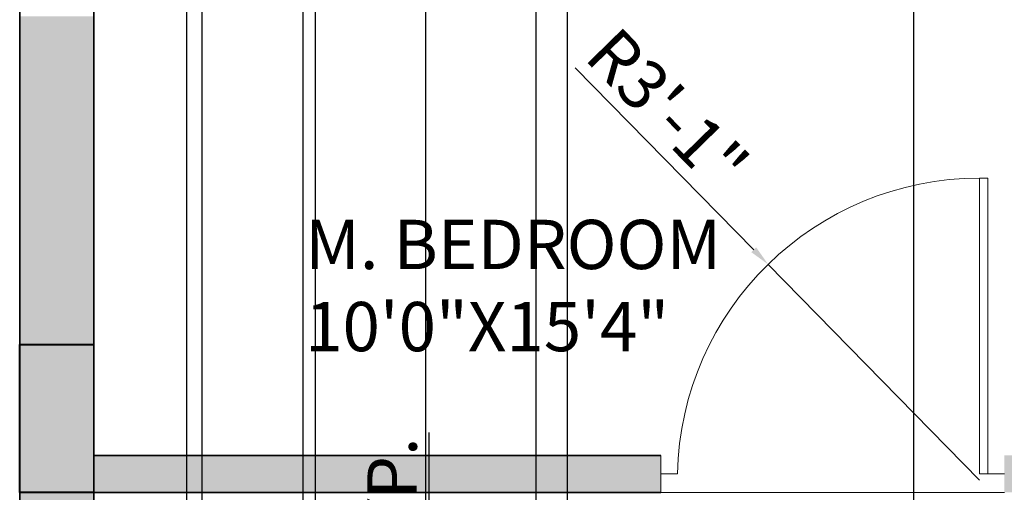
# Model space of a CAD drawing. Units: inches. Extents: x 2656 to 9931, y 1941 to 3068.
# Tile 5 of 46: x 2743 to 2863, y 2426 to 2484. Entities that reach past the tile are written whole.
import ezdxf

# ---------------------------------------------------------------- set-up
doc = ezdxf.new("R2010")
doc.units = ezdxf.units.IN
for name, color, linetype, lineweight in [('A-ANNO-DIMS', 2, 'Continuous', 18), ('A-AREA-IDEN', 7, 'Continuous', 18), ('A-COLS', 7, 'Continuous', 40), ('A-COLS-PATT', 146, 'Continuous', 13), ('A-DOOR', 3, 'Continuous', 18), ('A-WALL', 7, 'Continuous', 35), ('A-WALL-PATT', 251, 'Continuous', 13)]:
    doc.layers.add(name, color=color, linetype=linetype, lineweight=lineweight)
doc.styles.get("Standard").update_dxf_attribs({"font": 'arial.ttf'})
doc.dimstyles.new('ISO-25', dxfattribs={"dimtxt": 6, "dimasz": 2.5, "dimexe": 1.25, "dimexo": 0.625, "dimtad": 1, "dimdec": 0, "dimlunit": 3, "dimtxsty": 'Standard', "dimcen": 2.5, "dimadec": 0, "dimazin": 0, "dimtfac": 1, "dimtdec": 0, "dimtmove": 0, "dimatfit": 3, "dimfxl": 1, "dimarcsym": 0})

# ---------------------------------------------------------------- blocks, each defined once
blk = doc.blocks.new('DOOR-BEDROOM-DINING')
for p, q in [((39.78, 38.25), (38.78, 38.25)), ((38.78, 38.25), (38.78, 2.25)), ((39.78, 2.25), (39.78, 38.25)), ((0.03, 2.25), (2.03, 2.25)), ((38.78, 2.25), (39.78, 2.25)), ((41.78, 2.25), (39.78, 2.25)), ((0.03, 0), (41.78, 0))]:
    blk.add_line(p, q)
blk.add_arc((38.78, 1.5), 36.75, 90, 178.8304)
blk = doc.blocks.new('*D31')
at = {"layer": 'A-ANNO-DIMS', "color": 0, "lineweight": -2, "transparency": 16777216}
for p, q in [((2753.36, 2502.15), (2753.36, 2488.23)), ((2841.98, 2502.15), (2841.98, 2488.23)), ((2755.86, 2489.48), (2839.48, 2489.48)), ((2841.98, 2489.48), (2952.35, 2489.48))]:
    blk.add_line(p, q, dxfattribs=at)
at = {"layer": 'A-ANNO-DIMS', "color": 0, "transparency": 16777216}
for points in [[(2755.86, 2489.89), (2755.86, 2489.06), (2753.36, 2489.48)], [(2839.48, 2489.89), (2839.48, 2489.06), (2841.98, 2489.48)]]:
    blk.add_solid(points, dxfattribs=at)
at = {"layer": 'Defpoints', "color": 0, "transparency": 16777216}
for p in [(2753.36, 2502.77), (2841.98, 2502.77), (2841.98, 2489.48)]:
    blk.add_point(p, dxfattribs=at)
at = {"layer": 'A-ANNO-DIMS', "color": 0, "transparency": 16777216, "insert": (2898.41, 2493.21), "char_height": 6, "attachment_point": 5}
blk.add_mtext('DOUBLE BED 7\'-4 1/2" TYP.', dxfattribs=at)
blk = doc.blocks.new('*D62')
at = {"layer": 'A-ANNO-DIMS', "color": 0, "lineweight": -2, "transparency": 16777216}
for p, q in [((2792.93, 2374.42), (2792.93, 2433.38)), ((2791.71, 2374.42), (2794.18, 2374.42)), ((2792.93, 2365.48), (2792.93, 2371.92)), ((2791.71, 2362.98), (2794.18, 2362.98))]:
    blk.add_line(p, q, dxfattribs=at)
at = {"layer": 'A-ANNO-DIMS', "color": 0, "transparency": 16777216}
for points in [[(2792.52, 2371.92), (2793.35, 2371.92), (2792.93, 2374.42)], [(2792.52, 2365.48), (2793.35, 2365.48), (2792.93, 2362.98)]]:
    blk.add_solid(points, dxfattribs=at)
at = {"layer": 'Defpoints', "color": 0, "transparency": 16777216}
for p in [(2791.08, 2374.42), (2792.93, 2374.42), (2791.08, 2362.98)]:
    blk.add_point(p, dxfattribs=at)
at = {"layer": 'A-ANNO-DIMS', "color": 0, "transparency": 16777216, "insert": (2789.21, 2405.15), "char_height": 6, "attachment_point": 5, "rotation": 90}
blk.add_mtext('0\'-11 1/2" TYP.', dxfattribs=at)
blk = doc.blocks.new('*D113')
at = {"layer": 'A-ANNO-DIMS', "color": 0, "lineweight": -2, "transparency": 16777216}
for p, q in [((2752.16, 2300.73), (2752.16, 2674.45)), ((2809.77, 2300.73), (2809.77, 2674.45)), ((2754.66, 2673.2), (2807.27, 2673.2))]:
    blk.add_line(p, q, dxfattribs=at)
at = {"layer": 'A-ANNO-DIMS', "color": 0, "transparency": 16777216}
for points in [[(2754.66, 2673.62), (2754.66, 2672.78), (2752.16, 2673.2)], [(2807.27, 2673.62), (2807.27, 2672.78), (2809.77, 2673.2)]]:
    blk.add_solid(points, dxfattribs=at)
at = {"layer": 'Defpoints', "color": 0, "transparency": 16777216}
for p in [(2809.77, 2673.2), (2752.16, 2300.1), (2809.77, 2300.1)]:
    blk.add_point(p, dxfattribs=at)
at = {"layer": 'A-ANNO-DIMS', "color": 0, "transparency": 16777216, "insert": (2780.96, 2676.93), "char_height": 6, "attachment_point": 5}
blk.add_mtext('4\'-9 1/2"', dxfattribs=at)
blk = doc.blocks.new('*D114')
at = {"layer": 'A-ANNO-DIMS', "color": 0, "lineweight": -2, "transparency": 16777216}
for p, q in [((2809.77, 2300.73), (2809.77, 2674.45)), ((2851.88, 2300.73), (2851.88, 2674.45)), ((2812.27, 2673.2), (2849.38, 2673.2))]:
    blk.add_line(p, q, dxfattribs=at)
at = {"layer": 'A-ANNO-DIMS', "color": 0, "transparency": 16777216}
for points in [[(2812.27, 2673.62), (2812.27, 2672.78), (2809.77, 2673.2)], [(2849.38, 2673.62), (2849.38, 2672.78), (2851.88, 2673.2)]]:
    blk.add_solid(points, dxfattribs=at)
at = {"layer": 'Defpoints', "color": 0, "transparency": 16777216}
for p in [(2851.88, 2673.2), (2809.77, 2300.1), (2851.88, 2300.1)]:
    blk.add_point(p, dxfattribs=at)
at = {"layer": 'A-ANNO-DIMS', "color": 0, "transparency": 16777216, "insert": (2830.82, 2676.89), "char_height": 6, "attachment_point": 5}
blk.add_mtext('3\'-6"', dxfattribs=at)
blk = doc.blocks.new('*D129')
at = {"layer": 'A-ANNO-DIMS', "color": 0, "lineweight": -2, "transparency": 16777216}
for p, q in [((2752.16, 2601.15), (2752.16, 2009.27)), ((2777.59, 2557.74), (2777.59, 2009.27)), ((2754.66, 2010.52), (2775.09, 2010.52)), ((2777.59, 2010.52), (2811.37, 2010.52))]:
    blk.add_line(p, q, dxfattribs=at)
at = {"layer": 'A-ANNO-DIMS', "color": 0, "transparency": 16777216}
for points in [[(2754.66, 2010.94), (2754.66, 2010.11), (2752.16, 2010.52)], [(2775.09, 2010.94), (2775.09, 2010.11), (2777.59, 2010.52)]]:
    blk.add_solid(points, dxfattribs=at)
at = {"layer": 'Defpoints', "color": 0, "transparency": 16777216}
for p in [(2752.16, 2601.77), (2777.59, 2558.37), (2777.59, 2010.52)]:
    blk.add_point(p, dxfattribs=at)
at = {"layer": 'A-ANNO-DIMS', "color": 0, "transparency": 16777216, "insert": (2795.73, 2014.25), "char_height": 6, "attachment_point": 5}
blk.add_mtext('2\'-1 1/2"', dxfattribs=at)
blk = doc.blocks.new('*D132')
at = {"layer": 'A-ANNO-DIMS', "color": 0, "lineweight": -2, "transparency": 16777216}
for p, q in [((2763.47, 2366.56), (2763.47, 2674.45)), ((2805.96, 2366.56), (2805.96, 2674.45)), ((2765.97, 2673.2), (2803.46, 2673.2))]:
    blk.add_line(p, q, dxfattribs=at)
at = {"layer": 'A-ANNO-DIMS', "color": 0, "transparency": 16777216}
for points in [[(2765.97, 2673.62), (2765.97, 2672.78), (2763.47, 2673.2)], [(2803.46, 2673.62), (2803.46, 2672.78), (2805.96, 2673.2)]]:
    blk.add_solid(points, dxfattribs=at)
at = {"layer": 'Defpoints', "color": 0, "transparency": 16777216}
for p in [(2805.96, 2673.2), (2763.47, 2365.93), (2805.96, 2365.93)]:
    blk.add_point(p, dxfattribs=at)
at = {"layer": 'A-ANNO-DIMS', "color": 0, "transparency": 16777216, "insert": (2784.72, 2676.93), "char_height": 6, "attachment_point": 5}
blk.add_mtext('3\'-6 1/2"', dxfattribs=at)
blk = doc.blocks.new('*D134')
at = {"layer": 'A-ANNO-DIMS', "color": 0, "lineweight": -2, "transparency": 16777216}
for p, q in [((2752.16, 2300.73), (2752.16, 2674.45)), ((2763.47, 2347.43), (2763.47, 2674.45)), ((2754.66, 2673.2), (2760.97, 2673.2)), ((2763.47, 2673.2), (2801.81, 2673.2))]:
    blk.add_line(p, q, dxfattribs=at)
at = {"layer": 'A-ANNO-DIMS', "color": 0, "transparency": 16777216}
for points in [[(2754.66, 2673.62), (2754.66, 2672.78), (2752.16, 2673.2)], [(2760.97, 2673.62), (2760.97, 2672.78), (2763.47, 2673.2)]]:
    blk.add_solid(points, dxfattribs=at)
at = {"layer": 'Defpoints', "color": 0, "transparency": 16777216}
for p in [(2763.47, 2673.2), (2763.47, 2346.81), (2752.16, 2300.1)]:
    blk.add_point(p, dxfattribs=at)
at = {"layer": 'A-ANNO-DIMS', "color": 0, "transparency": 16777216, "insert": (2783.89, 2676.93), "char_height": 6, "attachment_point": 5}
blk.add_mtext('0\'-11 1/2"', dxfattribs=at)
blk = doc.blocks.new('*D136')
at = {"layer": 'A-ANNO-DIMS', "color": 0, "lineweight": -2, "transparency": 16777216}
for p, q in [((2765.36, 2375.04), (2765.36, 2674.45)), ((2779.14, 2375.04), (2779.14, 2674.45)), ((2767.86, 2673.2), (2776.64, 2673.2)), ((2779.14, 2673.2), (2798.28, 2673.2))]:
    blk.add_line(p, q, dxfattribs=at)
at = {"layer": 'A-ANNO-DIMS', "color": 0, "transparency": 16777216}
for points in [[(2767.86, 2673.62), (2767.86, 2672.78), (2765.36, 2673.2)], [(2776.64, 2673.62), (2776.64, 2672.78), (2779.14, 2673.2)]]:
    blk.add_solid(points, dxfattribs=at)
at = {"layer": 'Defpoints', "color": 0, "transparency": 16777216}
for p in [(2779.14, 2673.2), (2765.36, 2374.42), (2779.14, 2374.42)]:
    blk.add_point(p, dxfattribs=at)
at = {"layer": 'A-ANNO-DIMS', "color": 0, "transparency": 16777216, "insert": (2789.96, 2676.84), "char_height": 6, "attachment_point": 5}
blk.add_mtext('1\'-2"', dxfattribs=at)
blk = doc.blocks.new('*D137')
at = {"layer": 'A-ANNO-DIMS', "color": 0, "lineweight": -2, "transparency": 16777216}
for p, q in [((2779.14, 2375.04), (2779.14, 2674.45)), ((2792.52, 2375.04), (2792.52, 2674.45)), ((2781.64, 2673.2), (2790.02, 2673.2)), ((2792.52, 2673.2), (2825.63, 2673.2))]:
    blk.add_line(p, q, dxfattribs=at)
at = {"layer": 'A-ANNO-DIMS', "color": 0, "transparency": 16777216}
for points in [[(2781.64, 2673.62), (2781.64, 2672.78), (2779.14, 2673.2)], [(2790.02, 2673.62), (2790.02, 2672.78), (2792.52, 2673.2)]]:
    blk.add_solid(points, dxfattribs=at)
at = {"layer": 'Defpoints', "color": 0, "transparency": 16777216}
for p in [(2792.52, 2673.2), (2779.14, 2374.42), (2792.52, 2374.42)]:
    blk.add_point(p, dxfattribs=at)
at = {"layer": 'A-ANNO-DIMS', "color": 0, "transparency": 16777216, "insert": (2810.32, 2676.93), "char_height": 6, "attachment_point": 5}
blk.add_mtext('1\'-1 1/2"', dxfattribs=at)
blk = doc.blocks.new('*D184')
at = {"layer": 'A-ANNO-DIMS', "color": 0, "lineweight": -2, "transparency": 16777216}
for p, q in [((2810.7, 2477.79), (2832.41, 2455.64)), ((2859.88, 2427.6), (2834.16, 2453.85))]:
    blk.add_line(p, q, dxfattribs=at)
at = {"layer": 'A-ANNO-DIMS', "color": 0, "transparency": 16777216}
blk.add_solid([(2832.7, 2455.93), (2832.11, 2455.34), (2834.16, 2453.85)], dxfattribs=at)
at = {"layer": 'Defpoints', "color": 0, "transparency": 16777216}
for p in [(2834.16, 2453.85), (2859.88, 2427.6)]:
    blk.add_point(p, dxfattribs=at)
at = {"layer": 'A-ANNO-DIMS', "color": 0, "transparency": 16777216, "insert": (2821.36, 2472.18), "char_height": 6, "attachment_point": 5, "rotation": 314.4151}
blk.add_mtext('R3\'-1"', dxfattribs=at)

msp = doc.modelspace()

# ---------------------------------------------------------------- hatches: boundary and pattern name
at = {"layer": 'A-COLS-PATT'}
h = msp.add_hatch(color=256, dxfattribs=at)
h.dxf.hatch_style = 1
h.paths.add_polyline_path([(2752.16, 2623.6), (2743.16, 2623.6), (2743.16, 2605.6), (2752.16, 2605.6)])
h.paths.add_polyline_path([(2876.66, 2623.6), (2858.66, 2623.6), (2858.66, 2614.6), (2876.66, 2614.6)])
h.paths.add_polyline_path([(2998.16, 2623.6), (2989.16, 2623.6), (2989.16, 2614.6), (2989.16, 2605.6), (2998.16, 2605.6)])
h.paths.add_polyline_path([(2998.16, 2444.1), (2989.16, 2444.1), (2989.16, 2426.1), (2998.16, 2426.1)])
h.paths.add_polyline_path([(2876.66, 2444.1), (2867.66, 2444.1), (2867.66, 2426.1), (2876.66, 2426.1)])
h.paths.add_polyline_path([(2752.16, 2444.1), (2743.16, 2444.1), (2743.16, 2426.1), (2752.16, 2426.1)])
h.paths.add_polyline_path([(2752.16, 2300.1), (2743.16, 2300.1), (2743.16, 2282.1), (2752.16, 2282.1)])
h.paths.add_polyline_path([(2876.66, 2300.1), (2867.66, 2300.1), (2867.66, 2282.1), (2876.66, 2282.1)])
h.paths.add_polyline_path([(2998.16, 2300.1), (2989.16, 2300.1), (2989.16, 2282.1), (2998.16, 2282.1)])
h.paths.add_polyline_path([(2998.16, 2184.6), (2989.16, 2184.6), (2989.16, 2166.6), (2998.16, 2166.6)])
h.paths.add_polyline_path([(2876.66, 2175.6), (2858.66, 2175.6), (2858.66, 2166.6), (2876.66, 2166.6)])
h.paths.add_polyline_path([(2752.16, 2184.6), (2743.16, 2184.6), (2743.16, 2166.6), (2752.16, 2166.6)])
at = {"layer": 'A-WALL-PATT'}
h = msp.add_hatch(color=256, dxfattribs=at)
h.dxf.hatch_style = 1
h.paths.add_polyline_path([(2858.66, 2623.6), (2752.16, 2623.6), (2752.16, 2614.6), (2858.66, 2614.6)])
h.paths.add_polyline_path([(2893.09, 2623.6), (2876.66, 2623.6), (2876.66, 2614.6), (2893.09, 2614.6), (2893.09, 2619.1)])
h.paths.add_polyline_path([(2946.51, 2623.6), (2917.09, 2623.6), (2917.09, 2614.6), (2946.51, 2614.6), (2946.51, 2619.1)])
h.paths.add_polyline_path([(2989.16, 2623.6), (2970.51, 2623.6), (2970.51, 2614.6), (2989.16, 2614.6)])
h.paths.add_polyline_path([(2998.16, 2605.6), (2989.16, 2605.6), (2989.16, 2523.88), (2998.16, 2523.88)])
h.paths.add_polyline_path([(2935.16, 2614.6), (2930.66, 2614.6), (2930.66, 2554.6), (2876.66, 2554.6), (2876.66, 2565.34), (2872.16, 2565.34), (2872.16, 2444.1), (2876.66, 2444.1), (2876.66, 2550.1), (2946.47, 2550.1), (2946.47, 2554.6), (2935.16, 2554.6)])
h.paths.add_polyline_path([(2989.16, 2554.6), (2982.11, 2554.6), (2976.57, 2554.6), (2976.57, 2550.1), (2982.11, 2550.1), (2989.16, 2550.1)])
h.paths.add_polyline_path([(2876.66, 2614.6), (2872.16, 2614.6), (2872.16, 2595), (2876.66, 2595)], flags=0)
h.paths.add_polyline_path([(2752.16, 2605.6), (2743.16, 2605.6), (2743.16, 2544.03), (2752.16, 2544.03)])
h.paths.add_polyline_path([(2752.16, 2426.1), (2743.16, 2426.1), (2743.16, 2300.1), (2752.16, 2300.1)])
h.paths.add_polyline_path([(2821.13, 2430.6), (2752.16, 2430.6), (2752.16, 2426.1), (2821.13, 2426.1)])
h.paths.add_polyline_path([(2867.66, 2430.6), (2862.88, 2430.6), (2862.88, 2426.1), (2867.66, 2426.1)])
h.paths.add_polyline_path([(2752.16, 2484.03), (2747.66, 2484.03), (2743.16, 2484.03), (2743.16, 2444.1), (2752.16, 2444.1)])
h.paths.add_polyline_path([(2998.16, 2426.1), (2989.16, 2426.1), (2989.16, 2390.1), (2872.16, 2390.1), (2872.16, 2385.6), (2876.66, 2385.6), (2989.16, 2385.6), (2989.16, 2365.04), (2998.16, 2365.04)])
h.paths.add_polyline_path([(2998.16, 2463.88), (2993.66, 2463.88), (2989.16, 2463.88), (2989.16, 2444.1), (2998.16, 2444.1)])
h.paths.add_polyline_path([(2998.16, 2319.88), (2989.16, 2319.88), (2989.16, 2300.1), (2998.16, 2300.1)])
h.paths.add_polyline_path([(2998.16, 2282.1), (2989.16, 2282.1), (2989.16, 2253.6), (2982.06, 2253.6), (2982.06, 2249.1), (2989.16, 2249.1), (2998.16, 2249.1)])
h.paths.add_polyline_path([(2931.54, 2253.6), (2923.8, 2253.6), (2923.8, 2249.1), (2931.54, 2249.1)])
h.paths.add_polyline_path([(2876.66, 2282.1), (2872.16, 2282.1), (2872.16, 2184.6), (2872.16, 2175.6), (2876.66, 2175.6), (2876.66, 2249.1), (2888.32, 2249.1), (2888.32, 2251.35), (2888.32, 2253.6), (2876.66, 2253.6)])
h.paths.add_polyline_path([(2858.66, 2175.6), (2841.42, 2175.6), (2841.42, 2166.6), (2858.66, 2166.6)])
h.paths.add_polyline_path([(2785.06, 2171.1), (2785.06, 2175.6), (2752.16, 2175.6), (2752.16, 2166.6), (2785.06, 2166.6)])
h.paths.add_polyline_path([(2752.16, 2282.1), (2743.16, 2282.1), (2743.16, 2184.6), (2752.16, 2184.6)])
h.paths.add_polyline_path([(2809.77, 2300.1), (2752.16, 2300.1), (2752.16, 2295.6), (2809.77, 2295.6)])
h.paths.add_polyline_path([(2867.66, 2300.1), (2851.88, 2300.1), (2851.88, 2295.6), (2867.66, 2295.6)])

# ---------------------------------------------------------------- linework, layer by layer
at = {"layer": 'A-COLS'}
for p, q in [((2743.16, 2426.1), (2743.16, 2444.1)), ((2743.16, 2444.1), (2752.16, 2444.1)), ((2752.16, 2426.1), (2743.16, 2426.1))]:
    msp.add_line(p, q, dxfattribs=at)
at = {"layer": 'A-DOOR'}
msp.add_line((2821.13, 2430.6), (2821.13, 2426.1), dxfattribs=at)
at = {"layer": 'A-WALL'}
for p, q in [((2743.16, 2623.6), (2743.16, 2166.6)), ((2752.16, 2614.6), (2752.16, 2166.6)), ((2752.16, 2430.6), (2821.13, 2430.6)), ((2752.16, 2426.1), (2821.13, 2426.1))]:
    msp.add_line(p, q, dxfattribs=at)

# ---------------------------------------------------------------- block references
at = {"layer": 'A-DOOR'}
msp.add_blockref('DOOR-BEDROOM-DINING', (2821.1, 2426.1), dxfattribs=at)

# ---------------------------------------------------------------- texts
at = {"layer": 'A-AREA-IDEN', "insert": (2777.87, 2459.28), "char_height": 6, "attachment_point": 1}
msp.add_mtext_dynamic_manual_height_columns('M. BEDROOM\\P10\'0"X15\'4"', width=137.4726, gutter_width=12.5, heights=[0], dxfattribs=at)

# ---------------------------------------------------------------- dimensions: what is measured, and where the dimension line sits
at = {"layer": 'A-ANNO-DIMS'}
for base, p1, p2, picture, middle in [((2809.77, 2673.2), (2752.16, 2300.1), (2809.77, 2300.1), '*D113', (2780.96, 2676.93)), ((2763.47, 2673.2), (2752.16, 2300.1), (2763.47, 2346.81), '*D134', (2783.89, 2676.93)), ((2805.96, 2673.2), (2763.47, 2365.93), (2805.96, 2365.93), '*D132', (2784.72, 2676.93)), ((2792.52, 2673.2), (2779.14, 2374.42), (2792.52, 2374.42), '*D137', (2810.32, 2676.93)), ((2779.14, 2673.2), (2765.36, 2374.42), (2779.14, 2374.42), '*D136', (2789.96, 2676.84)), ((2851.88, 2673.2), (2809.77, 2300.1), (2851.88, 2300.1), '*D114', (2830.82, 2676.89)), ((2777.59, 2010.52), (2752.16, 2601.77), (2777.59, 2558.37), '*D129', (2795.73, 2014.25))]:
    dim = msp.add_linear_dim(base=base, p1=p1, p2=p2, dimstyle='ISO-25', override={"dimdec": 1, "dimlfac": 1, "dimrnd": 0, "dimzin": 1, "dimdsep": 46, "dimlunit": 4, "dimfrac": 2}, dxfattribs=at)
    dim.commit()
    dim.dimension.update_dxf_attribs({"geometry": picture, "text_midpoint": middle})
dim = msp.add_linear_dim(base=(2841.98, 2489.48), p1=(2753.36, 2502.77), p2=(2841.98, 2502.77), text='DOUBLE BED <> TYP.', dimstyle='ISO-25', override={"dimdec": 1, "dimlfac": 1, "dimrnd": 0, "dimzin": 1, "dimdsep": 46, "dimlunit": 4, "dimfrac": 2}, dxfattribs=at)
dim.commit()
dim.dimension.update_dxf_attribs({"geometry": '*D31', "text_midpoint": (2898.41, 2493.21)})
dim = msp.add_radius_dim(center=(2859.88, 2427.6), mpoint=(2834.16, 2453.85), dimstyle='ISO-25', override={"dimdec": 1, "dimlfac": 1, "dimrnd": 0, "dimzin": 1, "dimdsep": 46, "dimlunit": 4, "dimfrac": 2}, dxfattribs=at)
dim.commit()
dim.dimension.update_dxf_attribs({"geometry": '*D184', "text_midpoint": (2818.72, 2469.6), "dimtype": 164})
dim = msp.add_linear_dim(base=(2792.93, 2374.42), p1=(2791.08, 2362.98), p2=(2791.08, 2374.42), angle=90, text='<> TYP.', dimstyle='ISO-25', override={"dimdec": 1, "dimlfac": 1, "dimrnd": 0, "dimzin": 1, "dimdsep": 46, "dimlunit": 4, "dimfrac": 2}, dxfattribs=at)
dim.commit()
dim.dimension.update_dxf_attribs({"geometry": '*D62', "text_midpoint": (2789.21, 2405.15)})

doc.saveas('drawing.dxf')
